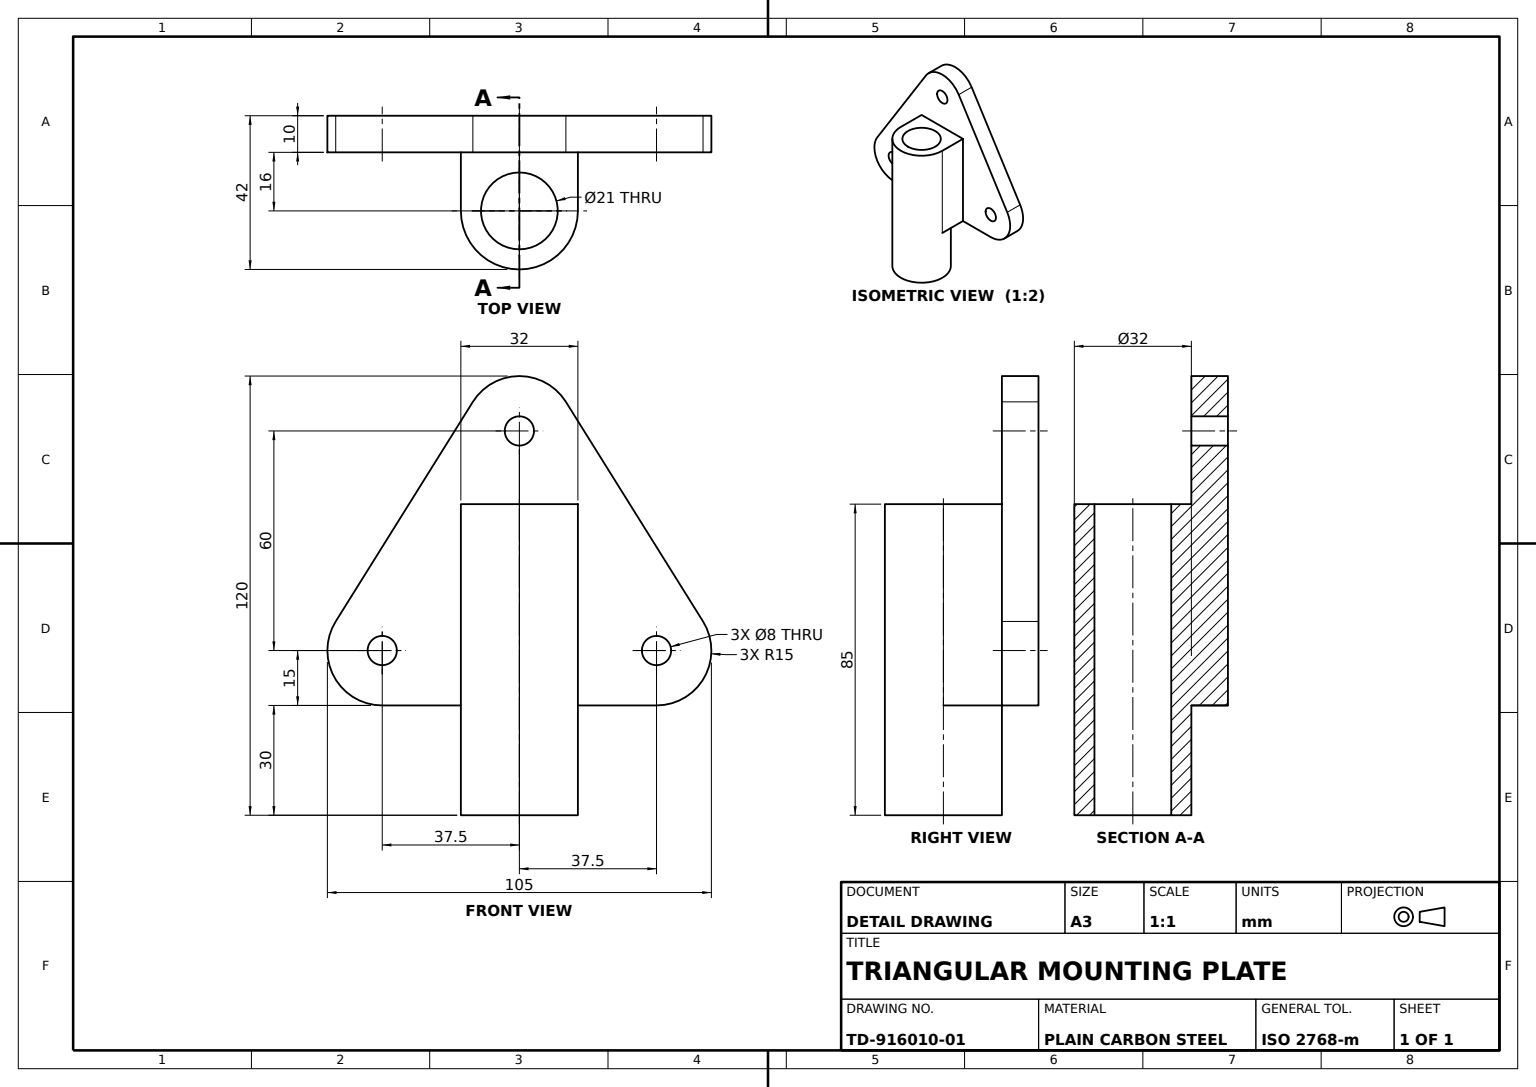
from build123d import *

# Parameters (mm, degrees)
TRIANGULAR_BASE_PLATE_DEPTH   = 10
TUBE_SUPPORT_BLOCK_PROFILE_W  = 16
TUBE_SUPPORT_BLOCK_PROFILE_H  = 10
TUBE_SUPPORT_BLOCK_DEPTH      = 55
SUPPORT_WEB_PROFILE_W         = 16
SUPPORT_WEB_PROFILE_H         = 6
SUPPORT_WEB_DEPTH             = 55
TUBE_PROFILE_32_R             = 16
ROUND_TUBE_32_DEPTH           = 55
TUBE_START                    = 30
TUBE_EXTENSION_PROFILE_32_R   = 16
TUBE_EXTENSION_32_DEPTH       = 30
TUBE_BORE_PROFILE_21_R        = 10.5
TUBE_BORE_21_DEPTH            = 85
MOUNTING_HOLES_PROFILE_3X_8_R = 4
MOUNTING_HOLES_3X_8_DEPTH     = 85


with BuildPart() as part:
    # Base Plate Profile → Triangular Base Plate (new body)
    with BuildSketch(Plane.XY):
        with BuildLine():
            Line((-50.21997456, -52.0500159), (-12.71997456, 7.9499841))
            ThreePointArc((-12.71997456, 7.9499841), (0, 15), (12.71997456, 7.9499841))
            Line((12.71997456, 7.9499841), (50.21997456, -52.0500159))
            ThreePointArc((50.21997456, -52.0500159), (50.619637219, -67.271527986), (37.5, -75))
            Line((37.5, -75), (-37.5, -75))
            ThreePointArc((-37.5, -75), (-50.619637219, -67.271527986), (-50.21997456, -52.0500159))
        make_face()
    extrude(amount=TRIANGULAR_BASE_PLATE_DEPTH)

    # Tube Support Block Profile → Tube Support Block (add)
    with BuildSketch(Plane.XZ.offset(75)):
        with Locations((-8, 15)):
            Rectangle(TUBE_SUPPORT_BLOCK_PROFILE_W, TUBE_SUPPORT_BLOCK_PROFILE_H)
        with Locations((8, 15)):
            Rectangle(TUBE_SUPPORT_BLOCK_PROFILE_W, TUBE_SUPPORT_BLOCK_PROFILE_H)
    extrude(amount=-TUBE_SUPPORT_BLOCK_DEPTH)

    # Support Web Profile → Support Web (add)
    with BuildSketch(Plane.XZ.offset(75)):
        with Locations((-8, 23)):
            Rectangle(SUPPORT_WEB_PROFILE_W, SUPPORT_WEB_PROFILE_H)
        with Locations((8, 23)):
            Rectangle(SUPPORT_WEB_PROFILE_W, SUPPORT_WEB_PROFILE_H)
    extrude(amount=-SUPPORT_WEB_DEPTH)

    # Tube Profile Ø32 → Round Tube Ø32 (add)
    with BuildSketch(Plane.XZ.offset(75)):
        with Locations((0, 26)):
            Circle(TUBE_PROFILE_32_R)
    extrude(amount=-ROUND_TUBE_32_DEPTH)

    # Tube Extension Profile Ø32 → Tube Extension Ø32 (add)
    with BuildSketch(Plane.XZ.offset(75).offset(TUBE_START)):
        with Locations(Location((0, 26, 0), (0, 0, 270))):
            Circle(TUBE_EXTENSION_PROFILE_32_R)
    extrude(amount=-TUBE_EXTENSION_32_DEPTH)

    # Tube Bore Profile Ø21 → Tube Bore Ø21 (cut)
    with BuildSketch(Plane.XZ.offset(105)):
        with Locations(Location((0, 26, 0), (0, 0, 270))):
            Circle(TUBE_BORE_PROFILE_21_R)
    extrude(amount=-TUBE_BORE_21_DEPTH, mode=Mode.SUBTRACT)

    # Mounting Holes Profile 3xØ8 → Mounting Holes 3xØ8 (cut)
    with BuildSketch(Plane.XY.offset(10)):
        Circle(MOUNTING_HOLES_PROFILE_3X_8_R)
        with Locations((-37.5, -60)):
            Circle(MOUNTING_HOLES_PROFILE_3X_8_R)
        with Locations((37.5, -60)):
            Circle(MOUNTING_HOLES_PROFILE_3X_8_R)
    extrude(amount=-MOUNTING_HOLES_3X_8_DEPTH, mode=Mode.SUBTRACT)


solid = part.part
